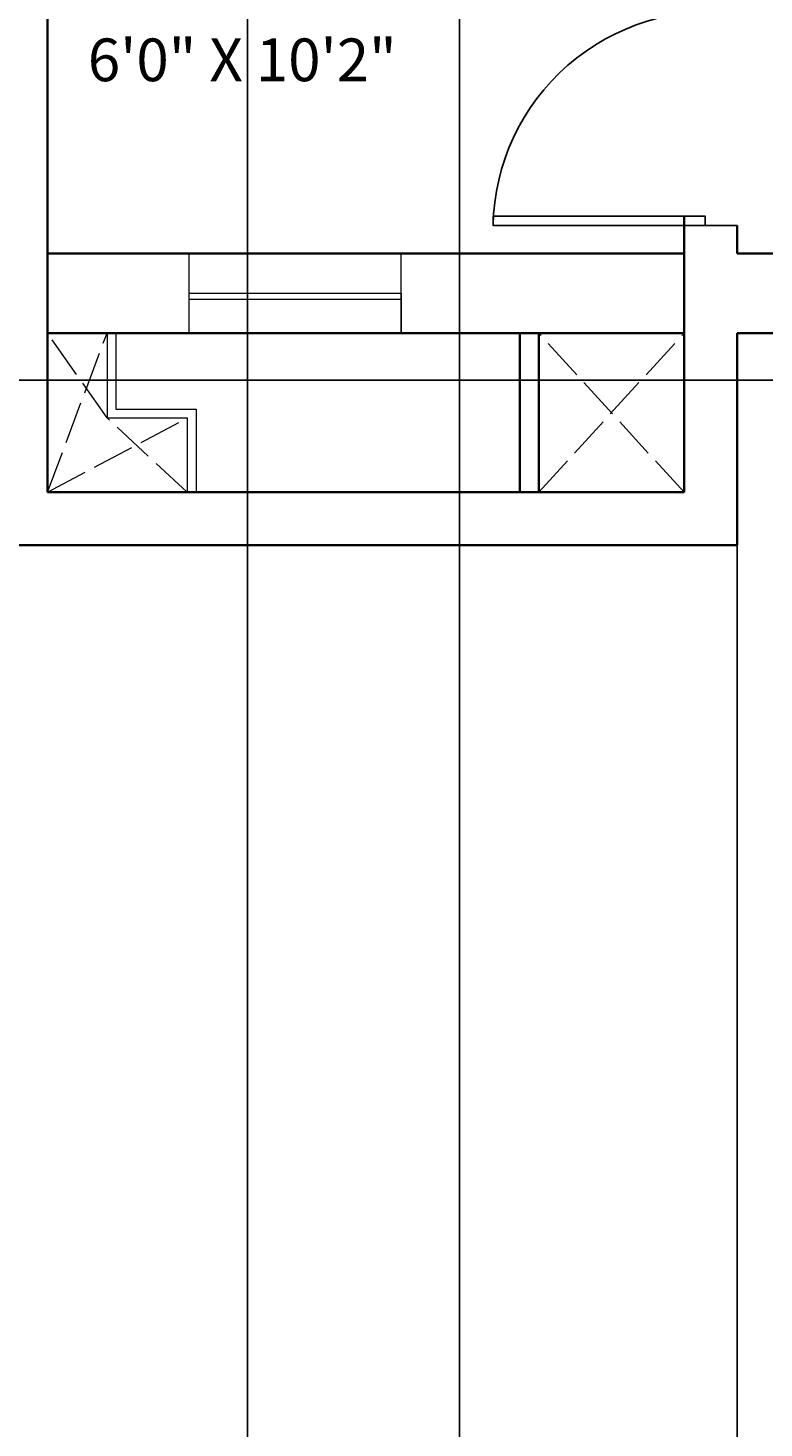
# Model space of a CAD drawing. Units: inches. Extents: x -61 to 1599, y -1316 to 257.
# Tile 80 of 204: x 323 to 407, y -565 to -407. Entities that reach past the tile are written whole.
import ezdxf

# ---------------------------------------------------------------- set-up
doc = ezdxf.new("R2010")
doc.units = ezdxf.units.IN
doc.header["$MEASUREMENT"] = 0
doc.linetypes.add('ACAD_ISO02W100', pattern=[15, 12, -3])
for name, color, linetype, lineweight in [('A-ANNO-DIMS', 2, 'Continuous', 18), ('A-AREA-IDEN', 1, 'Continuous', 18), ('A-FLOR-OPEN-HIDN', 8, 'ACAD_ISO02W100', 13), ('A-WALL-JAMB', 4, 'ACAD_ISO02W100', 25), ('DOORS', 2, 'Continuous', 25), ('WALLS', 4, 'Continuous', 35), ('WINDOWS', 220, 'Continuous', 18)]:
    doc.layers.add(name, color=color, linetype=linetype, lineweight=lineweight)
doc.styles.get("Standard").update_dxf_attribs({"font": 'arial.ttf'})
doc.dimstyles.get("Standard").update_dxf_attribs({"dimtxt": 0.18, "dimasz": 0.18, "dimexe": 0.18, "dimexo": 0.0625, "dimgap": 0.09, "dimtad": 0, "dimtih": 1, "dimtoh": 1, "dimdec": 0, "dimzin": 0, "dimdsep": 46, "dimlunit": 3, "dimtxsty": 'Standard', "dimcen": 0.09, "dimadec": 0, "dimazin": 0, "dimtfac": 1, "dimtdec": 0, "dimtofl": 0, "dimtmove": 0, "dimatfit": 3, "dimfxl": 1, "dimtolj": 1, "dimtzin": 0, "dimarcsym": 0})

# ---------------------------------------------------------------- blocks, each defined once
blk = doc.blocks.new('DOOR-SWING-24')
blk.add_line((0, 0), (0, 3.6))
blk.add_lwpolyline([(0, 0), (0, -24), (1.05, -24), (1.05, 0)], close=True)
blk.add_arc((-0.44, 0.62), 24.62, 271.0259, 6.9559)
blk = doc.blocks.new('WIN-24IN')
for p, q in [((0, 4.5), (0, 9)), ((0, 9), (0, 0)), ((24, 9), (24, 0)), ((0, 5.19), (24, 5.19)), ((0, 4.5), (24, 4.5))]:
    blk.add_line(p, q)
blk = doc.blocks.new('*D699')
at = {"layer": 'A-ANNO-DIMS', "color": 0, "lineweight": -2, "transparency": 16777216}
for p, q in [((835.64, -167.17), (-61.08, -167.17)), ((-60.9, -167.35), (-60.9, -306.73)), ((-60.9, -446.47), (-60.9, -307.09)), ((841.64, -446.65), (-61.08, -446.65))]:
    blk.add_line(p, q, dxfattribs=at)
at = {"layer": 'A-ANNO-DIMS', "color": 0, "transparency": 16777216}
for points in [[(-60.93, -167.35), (-60.87, -167.35), (-60.9, -167.17)], [(-60.93, -446.47), (-60.87, -446.47), (-60.9, -446.65)]]:
    blk.add_solid(points, dxfattribs=at)
at = {"layer": 'DEFPOINTS', "color": 0, "transparency": 16777216}
for p in [(835.7, -167.17), (-60.9, -446.65), (841.7, -446.65)]:
    blk.add_point(p, dxfattribs=at)
at = {"layer": 'A-ANNO-DIMS', "color": 0, "transparency": 16777216, "insert": (-60.9, -306.91), "char_height": 0.18, "attachment_point": 5}
blk.add_mtext('\\A1;279.5', dxfattribs=at)
blk = doc.blocks.new('*D702')
at = {"layer": 'A-ANNO-DIMS', "color": 0, "lineweight": -2, "transparency": 16777216}
for p, q in [((276.88, -616.88), (276.88, 257.46)), ((277.06, 257.28), (312.21, 257.28)), ((348.14, 257.28), (312.99, 257.28)), ((348.32, -616.88), (348.32, 257.46))]:
    blk.add_line(p, q, dxfattribs=at)
at = {"layer": 'A-ANNO-DIMS', "color": 0, "transparency": 16777216}
for points in [[(277.06, 257.31), (277.06, 257.25), (276.88, 257.28)], [(348.14, 257.31), (348.14, 257.25), (348.32, 257.28)]]:
    blk.add_solid(points, dxfattribs=at)
at = {"layer": 'DEFPOINTS', "color": 0, "transparency": 16777216}
for p in [(348.32, 257.28), (276.88, -616.94), (348.32, -616.94)]:
    blk.add_point(p, dxfattribs=at)
at = {"layer": 'A-ANNO-DIMS', "color": 0, "transparency": 16777216, "insert": (312.6, 257.28), "char_height": 0.18, "attachment_point": 5}
blk.add_mtext('\\A1;71.44', dxfattribs=at)
blk = doc.blocks.new('*D703')
at = {"layer": 'A-ANNO-DIMS', "color": 0, "lineweight": -2, "transparency": 16777216}
for p, q in [((372.32, -616.88), (372.32, 257.46)), ((372.5, 257.28), (413.7, 257.28)), ((455.65, 257.28), (414.45, 257.28)), ((455.83, -616.88), (455.83, 257.46))]:
    blk.add_line(p, q, dxfattribs=at)
at = {"layer": 'A-ANNO-DIMS', "color": 0, "transparency": 16777216}
for points in [[(372.5, 257.31), (372.5, 257.25), (372.32, 257.28)], [(455.65, 257.31), (455.65, 257.25), (455.83, 257.28)]]:
    blk.add_solid(points, dxfattribs=at)
at = {"layer": 'DEFPOINTS', "color": 0, "transparency": 16777216}
for p in [(455.83, 257.28), (372.32, -616.94), (455.83, -616.94)]:
    blk.add_point(p, dxfattribs=at)
at = {"layer": 'A-ANNO-DIMS', "color": 0, "transparency": 16777216, "insert": (414.08, 257.28), "char_height": 0.18, "attachment_point": 5}
blk.add_mtext('\\A1;83.51', dxfattribs=at)
blk = doc.blocks.new('*D710')
at = {"layer": 'A-ANNO-DIMS', "color": 0, "lineweight": -2, "transparency": 16777216}
for p, q in [((319.7, -465.39), (319.7, -1315.72)), ((403.7, -465.39), (403.7, -1315.72)), ((319.88, -1315.54), (361.48, -1315.54)), ((403.52, -1315.54), (361.92, -1315.54))]:
    blk.add_line(p, q, dxfattribs=at)
at = {"layer": 'A-ANNO-DIMS', "color": 0, "transparency": 16777216}
for points in [[(319.88, -1315.51), (319.88, -1315.57), (319.7, -1315.54)], [(403.52, -1315.51), (403.52, -1315.57), (403.7, -1315.54)]]:
    blk.add_solid(points, dxfattribs=at)
at = {"layer": 'DEFPOINTS', "color": 0, "transparency": 16777216}
for p in [(319.7, -465.32), (403.7, -465.32), (403.7, -1315.54)]:
    blk.add_point(p, dxfattribs=at)
at = {"layer": 'A-ANNO-DIMS', "color": 0, "transparency": 16777216, "insert": (361.7, -1315.54), "char_height": 0.18, "attachment_point": 5}
blk.add_mtext('\\A1;84', dxfattribs=at)

msp = doc.modelspace()

# ---------------------------------------------------------------- linework, layer by layer
at = {"layer": 'A-FLOR-OPEN-HIDN', "ltscale": 0.4}
for p, q in [((325.7028, -459.3229), (332.4306, -441.3229)), ((332.4306, -450.9215), (325.7028, -441.3229)), ((381.272, -459.3229), (397.7028, -441.3229)), ((397.7028, -459.3229), (381.272, -441.3229)), ((325.7028, -459.3229), (341.4965, -450.9215)), ((341.4965, -459.3229), (332.4306, -450.9215))]:
    msp.add_line(p, q, dxfattribs=at)
at = {"layer": 'A-FLOR-OPEN-HIDN'}
for p, q in [((332.4306, -441.3229), (332.4306, -450.9215)), ((333.4306, -441.3229), (333.4306, -449.9215)), ((332.4306, -450.9215), (341.4965, -450.9215)), ((333.4306, -449.9215), (342.4965, -449.9215)), ((341.4965, -450.9215), (341.4965, -459.3229)), ((342.4965, -449.9215), (342.4965, -459.3229))]:
    msp.add_line(p, q, dxfattribs=at)
at = {"layer": 'A-WALL-JAMB'}
msp.add_line((403.7028, -429.1414), (397.7028, -429.1414), dxfattribs=at)
at = {"layer": 'WALLS'}
for p, q in [((325.7028, -400.2211), (325.7028, -441.3229)), ((397.7028, -428.0914), (397.7028, -441.3229)), ((403.7028, -429.1414), (403.7028, -432.3229)), ((325.7028, -432.3229), (327.7028, -432.3229)), ((327.7028, -432.3229), (397.7028, -432.3229)), ((403.7028, -432.3229), (535.7028, -432.3229)), ((325.7028, -441.3229), (325.7028, -459.3229)), ((325.7028, -441.3229), (327.7028, -441.3229)), ((327.7028, -441.3229), (397.7028, -441.3229)), ((379.1436, -459.3229), (379.1436, -441.3229)), ((381.272, -459.3229), (381.272, -441.3229)), ((397.7028, -441.3229), (397.7028, -459.3229)), ((403.7028, -441.3229), (535.7028, -441.3229)), ((403.7028, -441.3229), (403.7028, -465.3229)), ((397.7028, -459.3229), (325.7028, -459.3229)), ((403.7028, -465.3229), (319.7028, -465.3229))]:
    msp.add_line(p, q, dxfattribs=at)

# ---------------------------------------------------------------- block references
at = {"layer": 'DOORS', "extrusion": (0, 0, -1), "zscale": -1, "rotation": 89.99999999999973}
msp.add_blockref('DOOR-SWING-24', (-400.1028, -429.1414), dxfattribs=at)
at = {"layer": 'WINDOWS', "rotation": 180}
msp.add_blockref('WIN-24IN', (365.7033, -432.3228), dxfattribs=at)

# ---------------------------------------------------------------- texts
at = {"layer": 'A-AREA-IDEN'}
msp.add_text('6\'0" X 10\'2"', height=4.832098, dxfattribs=at).set_placement((330.2598, -412.8182))

# ---------------------------------------------------------------- dimensions: what is measured, and where the dimension line sits
at = {"layer": 'A-ANNO-DIMS'}
for base, p1, p2, override, picture, middle in [((348.3201, 257.2771), (276.8825, -616.9446), (348.3201, -616.9446), {"dimdec": 2, "dimlfac": 1, "dimrnd": 0, "dimzin": 0, "dimdsep": 46, "dimlunit": 2}, '*D702', (312.6013, 257.2771)), ((455.8327, 257.2771), (372.3201, -616.9446), (455.8327, -616.9446), {"dimdec": 2, "dimlfac": 1, "dimrnd": 0, "dimzin": 0, "dimdsep": 46, "dimlunit": 2}, '*D703', (414.0764, 257.2771)), ((403.7028, -1315.5446), (319.7028, -465.3229), (403.7028, -465.3229), {"dimdec": 0, "dimlfac": 1, "dimrnd": 0, "dimzin": 0, "dimdsep": 46, "dimlunit": 2}, '*D710', (361.7028, -1315.5446))]:
    dim = msp.add_linear_dim(base=base, p1=p1, p2=p2, dimstyle='Standard', override=override, dxfattribs=at)
    dim.commit()
    dim.dimension.update_dxf_attribs({"geometry": picture, "text_midpoint": middle})
dim = msp.add_linear_dim(base=(-60.8972, -446.6462), p1=(835.7028, -167.169), p2=(841.7028, -446.6462), angle=90, dimstyle='Standard', override={"dimdec": 1, "dimlfac": 1, "dimrnd": 0, "dimzin": 0, "dimdsep": 46, "dimlunit": 2}, dxfattribs=at)
dim.commit()
dim.dimension.update_dxf_attribs({"geometry": '*D699', "text_midpoint": (-60.8972, -306.9076)})

doc.saveas('drawing.dxf')
